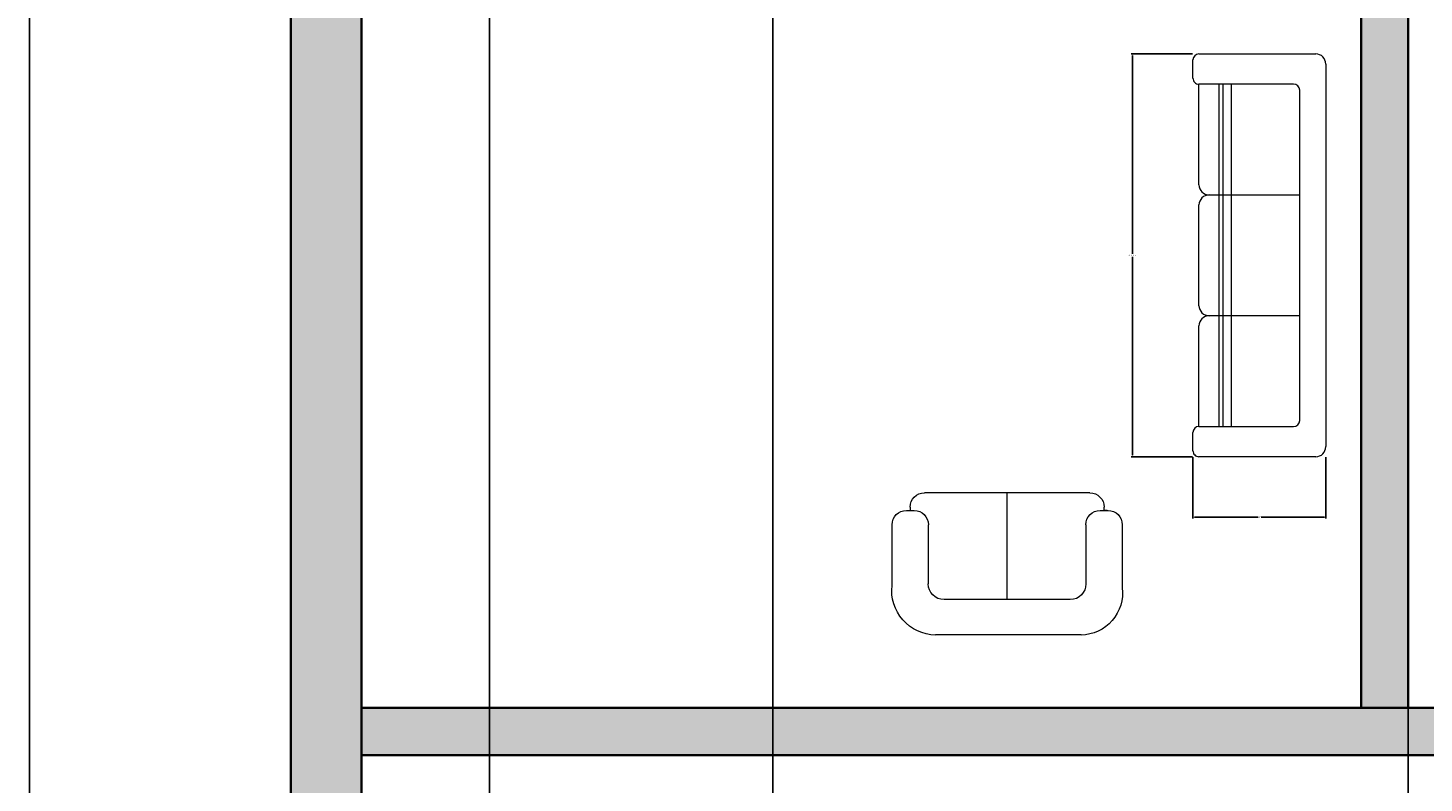
# Model space of a CAD drawing. Units: inches. Extents: x 2070 to 4408, y 1595 to 4269.
# Tile 2 of 20: x 2070 to 2247, y 1739 to 1835. Entities that reach past the tile are written whole.
import ezdxf

# ---------------------------------------------------------------- set-up
doc = ezdxf.new("R2010")
doc.units = ezdxf.units.IN
for name, color, linetype, lineweight in [('A-ANNO-DIMS', 2, 'Continuous', 18), ('A-FURN', 8, 'Continuous', 18), ('A-WALL', 7, 'Continuous', 35)]:
    doc.layers.add(name, color=color, linetype=linetype, lineweight=lineweight)
doc.layers.add('A-WALL-PATT', color=18, linetype='Continuous', lineweight=13, true_color=0x000000)
doc.styles.get("Standard").update_dxf_attribs({"font": 'arial.ttf'})
doc.dimstyles.get("Standard").update_dxf_attribs({"dimtxt": 0.18, "dimasz": 0.18, "dimexe": 0.18, "dimexo": 0.0625, "dimgap": 0.09, "dimtad": 0, "dimtih": 1, "dimtoh": 1, "dimdec": 4, "dimzin": 0, "dimdsep": 46, "dimtxsty": 'Standard', "dimcen": 0.09, "dimadec": 0, "dimazin": 0, "dimtfac": 1, "dimtdec": 4, "dimtofl": 0, "dimtmove": 0, "dimatfit": 3, "dimfxl": 1, "dimtolj": 1, "dimtzin": 0, "dimarcsym": 0})

# ---------------------------------------------------------------- blocks, each defined once
blk = doc.blocks.new('A$C05BA3A2B')
for p, q in [((0.05, 0.6596), (1.95, 0.6596)), ((0.05, 0.6596), (1.95, 0.6596)), ((0.05, 0.6596), (1.95, 0.6596)), ((0, 0.03), (0, 0.6096)), ((0, 0.03), (0, 0.6096)), ((0, 0.03), (0, 0.6096)), ((2, 0.6096), (2, 0.03)), ((2, 0.6096), (2, 0.03)), ((2, 0.6096), (2, 0.03)), ((0.15, 0.5), (0.15, 0.03)), ((0.15, 0.5), (0.15, 0.03)), ((0.15, 0.5), (0.15, 0.03)), ((1.82, 0.53), (0.18, 0.53)), ((1.82, 0.53), (0.18, 0.53)), ((1.82, 0.53), (0.18, 0.53)), ((0.7, 0.08), (0.7, 0.53)), ((0.7, 0.08), (0.7, 0.53)), ((0.7, 0.08), (0.7, 0.53)), ((1.3, 0.53), (1.3, 0.08)), ((1.3, 0.53), (1.3, 0.08)), ((1.3, 0.53), (1.3, 0.08)), ((1.85, 0.03), (1.85, 0.5)), ((1.85, 0.03), (1.85, 0.5)), ((1.85, 0.03), (1.85, 0.5)), ((1.85, 0.1908), (0.15, 0.1908)), ((1.85, 0.1908), (0.15, 0.1908)), ((1.85, 0.1908), (0.15, 0.1908)), ((1.85, 0.1508), (0.15, 0.1508)), ((1.85, 0.1508), (0.15, 0.1508)), ((1.85, 0.1508), (0.15, 0.1508)), ((1.85, 0.1308), (0.15, 0.1308)), ((1.85, 0.1308), (0.15, 0.1308)), ((1.85, 0.1308), (0.15, 0.1308)), ((0.12, 0), (0.03, 0)), ((0.12, 0), (0.03, 0)), ((0.12, 0), (0.03, 0)), ((0.65, 0.03), (0.15, 0.03)), ((0.65, 0.03), (0.15, 0.03)), ((0.65, 0.03), (0.15, 0.03)), ((1.25, 0.03), (0.75, 0.03)), ((1.25, 0.03), (0.75, 0.03)), ((1.25, 0.03), (0.75, 0.03)), ((1.85, 0.03), (1.35, 0.03)), ((1.85, 0.03), (1.35, 0.03)), ((1.85, 0.03), (1.35, 0.03)), ((1.97, 0), (1.88, 0)), ((1.97, 0), (1.88, 0)), ((1.97, 0), (1.88, 0))]:
    blk.add_line(p, q)
for centre, radius, start, end in [((0.05, 0.6096), 0.05, 90, 180), ((0.05, 0.6096), 0.05, 90, 180), ((0.05, 0.6096), 0.05, 90, 180), ((1.95, 0.6096), 0.05, 0, 90), ((1.95, 0.6096), 0.05, 0, 90), ((1.95, 0.6096), 0.05, 0, 90), ((0.18, 0.5), 0.03, 90, 180), ((0.18, 0.5), 0.03, 90, 180), ((0.18, 0.5), 0.03, 90, 180), ((1.82, 0.5), 0.03, 0, 90), ((1.82, 0.5), 0.03, 0, 90), ((1.82, 0.5), 0.03, 0, 90), ((0.65, 0.08), 0.05, 270, 0), ((0.65, 0.08), 0.05, 270, 0), ((0.65, 0.08), 0.05, 270, 0), ((0.75, 0.08), 0.05, 180, 270), ((0.75, 0.08), 0.05, 180, 270), ((0.75, 0.08), 0.05, 180, 270), ((1.25, 0.08), 0.05, 270, 0), ((1.25, 0.08), 0.05, 270, 0), ((1.25, 0.08), 0.05, 270, 0), ((1.35, 0.08), 0.05, 180, 270), ((1.35, 0.08), 0.05, 180, 270), ((1.35, 0.08), 0.05, 180, 270), ((0.03, 0.03), 0.03, 180, 270), ((0.03, 0.03), 0.03, 180, 270), ((0.03, 0.03), 0.03, 180, 270), ((0.12, 0.03), 0.03, 270, 0), ((0.12, 0.03), 0.03, 270, 0), ((0.12, 0.03), 0.03, 270, 0), ((1.88, 0.03), 0.03, 180, 270), ((1.88, 0.03), 0.03, 180, 270), ((1.88, 0.03), 0.03, 180, 270), ((1.97, 0.03), 0.03, 270, 0), ((1.97, 0.03), 0.03, 270, 0), ((1.97, 0.03), 0.03, 270, 0)]:
    blk.add_arc(centre, radius, start, end)
blk = doc.blocks.new('A$C6D011943')
for p, q in [((1.448, 1.089), (0.332, 1.089)), ((1.364, 0.818), (0.398, 0.818)), ((0.881, 0.818), (0.881, 0)), ((0, 0.709), (0, 0.247)), ((0.278, 0.697), (0.278, 0.244)), ((1.485, 0.244), (1.485, 0.697)), ((1.762, 0.247), (1.762, 0.727)), ((0.109, 0.136), (0.169, 0.136)), ((0.139, 0.109), (0.139, 0.136)), ((1.593, 0.136), (1.654, 0.136)), ((1.648, 0.136), (1.623, 0.136)), ((1.623, 0.109), (1.623, 0.136)), ((1.515, 0), (0.247, 0))]:
    blk.add_line(p, q)
for centre, radius, start, end in [((0.339, 0.748), 0.342, 91.2564, 186.501), ((1.441, 0.766), 0.324, 353.159, 88.6697), ((0.398, 0.697), 0.121, 90, 180), ((1.364, 0.697), 0.121, 0, 90), ((0.109, 0.244), 0.109, 180, 270), ((0.169, 0.244), 0.109, 270, 0), ((1.593, 0.244), 0.109, 180, 270), ((1.654, 0.244), 0.109, 270, 0), ((0.247, 0.109), 0.109, 180, 270), ((1.515, 0.109), 0.109, 270, 0)]:
    blk.add_arc(centre, radius, start, end)
blk = doc.blocks.new('*D19')
at = {"layer": 'A-ANNO-DIMS', "color": 0, "lineweight": -2, "transparency": 16777216}
for p, q in [((2217.78, 1831.51), (2209.98, 1831.51)), ((2210.16, 1831.33), (2210.16, 1806.1)), ((2210.16, 1780.51), (2210.16, 1805.73)), ((2217.78, 1780.33), (2209.98, 1780.33))]:
    blk.add_line(p, q, dxfattribs=at)
at = {"layer": 'A-ANNO-DIMS', "color": 0, "transparency": 16777216}
for points in [[(2210.13, 1831.33), (2210.19, 1831.33), (2210.16, 1831.51)], [(2210.13, 1780.51), (2210.19, 1780.51), (2210.16, 1780.33)]]:
    blk.add_solid(points, dxfattribs=at)
at = {"layer": 'Defpoints', "color": 0, "transparency": 16777216}
for p in [(2217.84, 1831.51), (2210.16, 1780.33), (2217.84, 1780.33)]:
    blk.add_point(p, dxfattribs=at)
at = {"layer": 'A-ANNO-DIMS', "color": 0, "transparency": 16777216, "insert": (2210.16, 1805.92), "char_height": 0.18, "attachment_point": 5}
blk.add_mtext('\\A1;SETTEE 51', dxfattribs=at)
blk = doc.blocks.new('*D20')
at = {"layer": 'A-ANNO-DIMS', "color": 0, "lineweight": -2, "transparency": 16777216}
for p, q in [((2217.84, 1780.26), (2217.84, 1772.47)), ((2234.72, 1780.26), (2234.72, 1772.47)), ((2218.02, 1772.65), (2226.07, 1772.65)), ((2234.54, 1772.65), (2226.49, 1772.65))]:
    blk.add_line(p, q, dxfattribs=at)
at = {"layer": 'A-ANNO-DIMS', "color": 0, "transparency": 16777216}
for points in [[(2218.02, 1772.68), (2218.02, 1772.62), (2217.84, 1772.65)], [(2234.54, 1772.68), (2234.54, 1772.62), (2234.72, 1772.65)]]:
    blk.add_solid(points, dxfattribs=at)
at = {"layer": 'Defpoints', "color": 0, "transparency": 16777216}
for p in [(2217.84, 1780.33), (2234.72, 1780.33), (2234.72, 1772.65)]:
    blk.add_point(p, dxfattribs=at)
at = {"layer": 'A-ANNO-DIMS', "color": 0, "transparency": 16777216, "insert": (2226.28, 1772.65), "char_height": 0.18, "attachment_point": 5}
blk.add_mtext('\\A1;17', dxfattribs=at)
blk = doc.blocks.new('*D24')
at = {"layer": 'A-ANNO-DIMS', "color": 0, "lineweight": -2, "transparency": 16777216}
for p, q in [((2103.13, 2291.4), (2069.84, 2291.4)), ((2070.02, 2291.22), (2070.02, 1960.08)), ((2070.02, 1628.58), (2070.02, 1959.72)), ((2336.13, 1628.4), (2069.84, 1628.4))]:
    blk.add_line(p, q, dxfattribs=at)
at = {"layer": 'A-ANNO-DIMS', "color": 0, "transparency": 16777216}
for points in [[(2069.99, 2291.22), (2070.05, 2291.22), (2070.02, 2291.4)], [(2069.99, 1628.58), (2070.05, 1628.58), (2070.02, 1628.4)]]:
    blk.add_solid(points, dxfattribs=at)
at = {"layer": 'Defpoints', "color": 0, "transparency": 16777216}
for p in [(2070.02, 2291.4), (2103.2, 2291.4), (2336.2, 1628.4)]:
    blk.add_point(p, dxfattribs=at)
at = {"layer": 'A-ANNO-DIMS', "color": 0, "transparency": 16777216, "insert": (2070.02, 1959.9), "char_height": 0.18, "attachment_point": 5}
blk.add_mtext('\\A1;663', dxfattribs=at)
blk = doc.blocks.new('*D29')
at = {"layer": 'A-ANNO-DIMS', "color": 0, "lineweight": -2, "transparency": 16777216}
for p, q in [((2128.44, 2150.34), (2128.44, 1595.04)), ((2164.44, 2150.34), (2164.44, 1595.04)), ((2128.62, 1595.22), (2146.22, 1595.22)), ((2164.26, 1595.22), (2146.65, 1595.22))]:
    blk.add_line(p, q, dxfattribs=at)
at = {"layer": 'A-ANNO-DIMS', "color": 0, "transparency": 16777216}
for points in [[(2128.62, 1595.25), (2128.62, 1595.19), (2128.44, 1595.22)], [(2164.26, 1595.25), (2164.26, 1595.19), (2164.44, 1595.22)]]:
    blk.add_solid(points, dxfattribs=at)
at = {"layer": 'Defpoints', "color": 0, "transparency": 16777216}
for p in [(2128.44, 2150.4), (2164.44, 2150.4), (2164.44, 1595.22)]:
    blk.add_point(p, dxfattribs=at)
at = {"layer": 'A-ANNO-DIMS', "color": 0, "transparency": 16777216, "insert": (2146.44, 1595.22), "char_height": 0.18, "attachment_point": 5}
blk.add_mtext('\\A1;36', dxfattribs=at)
blk = doc.blocks.new('*D32')
at = {"layer": 'A-ANNO-DIMS', "color": 0, "lineweight": -2, "transparency": 16777216}
for p, q in [((2245.2, 2230.58), (2245.2, 1595.04)), ((2340.2, 2230.58), (2340.2, 1595.04)), ((2245.38, 1595.22), (2292.48, 1595.22)), ((2340.02, 1595.22), (2292.92, 1595.22))]:
    blk.add_line(p, q, dxfattribs=at)
at = {"layer": 'A-ANNO-DIMS', "color": 0, "transparency": 16777216}
for points in [[(2245.38, 1595.25), (2245.38, 1595.19), (2245.2, 1595.22)], [(2340.02, 1595.25), (2340.02, 1595.19), (2340.2, 1595.22)]]:
    blk.add_solid(points, dxfattribs=at)
at = {"layer": 'Defpoints', "color": 0, "transparency": 16777216}
for p in [(2245.2, 2230.65), (2340.2, 2230.65), (2340.2, 1595.22)]:
    blk.add_point(p, dxfattribs=at)
at = {"layer": 'A-ANNO-DIMS', "color": 0, "transparency": 16777216, "insert": (2292.7, 1595.22), "char_height": 0.18, "attachment_point": 5}
blk.add_mtext('\\A1;95', dxfattribs=at)

msp = doc.modelspace()

# ---------------------------------------------------------------- hatches: boundary and pattern name
at = {"layer": 'A-WALL-PATT'}
h = msp.add_hatch(color=256, dxfattribs=at)
h.dxf.hatch_style = 1
h.paths.add_polyline_path([(2346.196, 2218.3995), (2346.196, 2282.3995), (2340.196, 2282.3995), (2340.196, 2212.3995), (2345.5866, 2212.3995), (2346.196, 2212.3995)], flags=0)
h.paths.add_polyline_path([(2245.196, 2282.3995), (2239.196, 2282.3995), (2239.196, 2186.3995), (2244.5866, 2186.3995), (2245.196, 2186.3995)], flags=0)
h.paths.add_polyline_path([(2340.196, 2230.6455), (2245.196, 2230.6455), (2245.196, 2224.6455), (2340.196, 2224.6455)], flags=0)
h.paths.add_polyline_path([(2245.196, 2150.3995), (2239.196, 2150.3995), (2164.4362, 2150.3995), (2164.4362, 2144.3995), (2239.196, 2144.3995), (2239.196, 2086.3995), (2239.196, 2067.2711), (2244.5866, 2067.2711), (2245.196, 2067.2711), (2245.196, 2144.3995)], flags=0)
h.paths.add_polyline_path([(2346.196, 2176.3995), (2340.196, 2176.3995), (2340.196, 2086.3995), (2346.196, 2086.3995), (2346.196, 2125.318)], flags=0)
h.paths.add_polyline_path([(2446.196, 2086.3995), (2346.196, 2086.3995), (2340.196, 2086.3995), (2340.196, 2080.3995), (2446.196, 2080.3995)], flags=0)
h.paths.add_polyline_path([(2455.196, 2291.3995), (2103.196, 2291.3995), (2103.196, 1699.3995), (2336.196, 1699.3995), (2336.196, 1628.3995), (2345.196, 1628.3995), (2446.196, 1628.3995), (2454.8846, 1628.3995), (2454.8846, 1699.3995)])
h.paths.add_polyline_path([(2446.196, 2282.3995), (2446.196, 2218.3995), (2446.196, 2212.3995), (2446.196, 2086.3995), (2446.196, 2080.3995), (2446.196, 1708.3995), (2446.196, 1637.3995), (2345.196, 1637.3995), (2345.196, 1699.3995), (2345.196, 1708.3995), (2336.196, 1708.3995), (2112.196, 1708.3995), (2112.196, 2282.3995), (2239.196, 2282.3995), (2245.196, 2282.3995), (2356.196, 2282.3995)], flags=16)
h.paths.add_polyline_path([(2245.196, 2150.3995), (2245.196, 2144.3995), (2245.196, 2067.2711), (2244.5866, 2067.2711), (2239.196, 2067.2711), (2239.196, 2065.6988), (2203.2929, 2065.6988, 0.40145271), (2239.196, 2031.3337), (2244.5866, 2031.3337), (2245.196, 2031.2711), (2245.196, 1924.1525), (2239.196, 1924.1525), (2239.196, 1922.5803), (2203.2929, 1922.5803, 0.40145271), (2239.196, 1888.2151), (2244.5866, 1888.2151), (2245.196, 1888.1525), (2245.196, 1748.3995), (2339.196, 1748.4621, -0.40145271), (2303.2929, 1782.8272), (2303.2585, 1782.8272), (2303.2585, 1784.3995), (2339.196, 1784.3995), (2339.196, 1877.2067), (2291.196, 1877.2067), (2291.196, 1883.2067), (2291.196, 1946.3995), (2291.196, 1952.3995), (2291.196, 2086.3995), (2297.196, 2086.3995), (2302.196, 2086.3995), (2302.196, 2081.0259), (2303.7633, 2081.0259), (2303.7633, 2080.3995), (2338.0148, 2080.3995, 0.00437129), (2338.0203, 2081.0259), (2338.0203, 2086.3995), (2340.196, 2086.3995), (2340.196, 2176.4621), (2345.5866, 2176.4621, 0.40145271), (2381.4896, 2210.8272), (2345.5866, 2210.8272), (2345.5866, 2212.3995), (2340.196, 2212.3995), (2340.196, 2224.6455), (2245.196, 2224.6455), (2245.196, 2186.3995), (2244.5866, 2186.3995), (2239.196, 2186.3995), (2239.196, 2184.8272), (2203.2929, 2184.8272, 0.40145271), (2239.196, 2150.4621), (2244.5866, 2150.4621)], flags=0)
h.paths.add_polyline_path([(2346.196, 2282.3995), (2346.196, 2218.3995), (2377.1813, 2218.3995), (2377.1813, 2212.3995), (2346.196, 2212.3995), (2345.5866, 2212.3995), (2340.196, 2212.3995), (2340.196, 2224.6455), (2245.196, 2224.6455), (2245.196, 2230.6455), (2245.196, 2282.3995), (2292.696, 2256.5225), (2340.196, 2282.3995)], flags=0)
h.paths.add_polyline_path([(2346.196, 2086.3995), (2340.196, 2086.3995), (2340.196, 2080.3995), (2446.196, 2080.3995), (2431.196, 2016.3995), (2446.196, 1952.3995), (2412.196, 1952.3995), (2412.196, 2080.3995), (2340.196, 2080.3995), (2340.196, 2086.3995), (2340.196, 2176.3995), (2346.196, 2176.3995), (2346.196, 2125.318)], flags=0)
h.paths.add_polyline_path([(2186.508, 2270.0471, -0.03755288), (2186.9712, 2269.8581), (2186.9164, 2270.112, -0.02759121)], flags=0)
h.paths.add_polyline_path([(2183.955, 2273.7766, 1), (2188.2945, 2273.7766, 1)], flags=0)
h.paths.add_polyline_path([(2142.5261, 2274.6158, -0.03707541), (2142.5672, 2275.1696), (2142.5672, 2276.826), (2119.8759, 2276.826), (2119.8759, 2263.0962), (2140.4332, 2263.0962), (2142.5672, 2263.0962), (2142.5672, 2274.0621, -0.03707541)], flags=0)
h.paths.add_polyline_path([(2209.8974, 2263.0962), (2209.8974, 2262.2079), (2190.8042, 2262.2079), (2190.8042, 2263.0962)], flags=0)
h.paths.add_polyline_path([(2210.6382, 2276.1833), (2210.6382, 2263.9844), (2190.2185, 2263.9844), (2190.2185, 2276.1833)], flags=0)
h.paths.add_polyline_path([(2188.4362, 2273.7766, -1), (2183.8133, 2273.7766, -1)], flags=0)
h.paths.add_polyline_path([(2245.196, 2150.3995), (2245.196, 2144.3995), (2245.196, 2067.2711), (2239.196, 2067.2711), (2239.196, 2080.3995), (2172.196, 2080.3995), (2172.196, 2000.3995), (2239.196, 2000.3995), (2239.196, 1940.3995), (2159.0187, 1940.3995), (2123.0187, 1940.3995), (2112.196, 1940.3995), (2112.196, 1946.3995), (2123.0187, 1946.3995), (2123.0187, 1982.2238), (2124.586, 1982.2238), (2124.586, 1982.1895, -0.40145271), (2158.8429, 1946.3995), (2159.0187, 1946.3995), (2239.196, 1946.3995), (2239.196, 1994.3995), (2112.196, 1994.3995), (2112.196, 2000.3995), (2139.196, 2040.3995), (2112.196, 2080.3995), (2112.196, 2086.3995), (2239.196, 2086.3995), (2239.196, 2144.3995), (2209.5809, 2144.3995), (2209.5809, 2136.3995), (2203.0809, 2136.3995), (2205.0809, 2130.3996, -0.70257121), (2199.081, 2116.3995, -0.70256205), (2193.0809, 2130.3994), (2195.0809, 2136.3995), (2192.0809, 2136.3995), (2192.0809, 2134.8995), (2189.0809, 2134.8995), (2189.0809, 2135.8995), (2191.0809, 2135.8995), (2191.0809, 2136.3995), (2188.5809, 2136.3995), (2188.5809, 2144.3995), (2164.2481, 2144.3995, -0.39385849), (2130.0035, 2109.5491), (2130.0035, 2109.5147), (2128.4362, 2109.5147), (2128.4362, 2144.3995), (2112.196, 2144.3995), (2112.196, 2150.3995), (2128.4362, 2150.3995), (2128.4362, 2150.7127), (2164.4362, 2150.7127), (2164.4362, 2150.3995), (2239.196, 2150.3995)], flags=0)
h.paths.add_polyline_path([(2188.2075, 2266.8735), (2188.2075, 2211.8632, -0.41421356), (2185.4833, 2209.1391), (2146.7995, 2209.1391, -0.41421356), (2144.0754, 2211.8632), (2144.0754, 2266.8735, -0.41421356), (2146.7995, 2269.5976), (2185.4833, 2269.5976, -0.41421356)], flags=0)
h.paths.add_polyline_path([(2185.0844, 2273.7766, -1), (2187.1651, 2273.7766, -1)], flags=0)
h.paths.add_polyline_path([(2182.0486, 2259.2932), (2168.0953, 2259.2932), (2168.0953, 2260.8424), (2163.7261, 2260.8424), (2163.7261, 2259.2932), (2149.7727, 2259.2932), (2149.7727, 2266.3352), (2163.7261, 2266.3352), (2163.7261, 2261.9839), (2168.0953, 2261.9839), (2168.0953, 2266.3352), (2182.0486, 2266.3352)], flags=0)
h.paths.add_polyline_path([(2148.2585, 2250.2051), (2153.0615, 2241.8861, 0.39807048)], flags=0)
h.paths.add_polyline_path([(2162.7572, 2247.2885), (2153.1461, 2241.7396), (2148.1083, 2250.4653), (2157.7194, 2256.0142)], flags=0)
h.paths.add_polyline_path([(2162.6726, 2247.4351, -0.39286196), (2157.8415, 2255.6313), (2157.6431, 2255.6313), (2157.8696, 2255.7541)], flags=0)
h.paths.add_polyline_path([(2164.2604, 2145.339), (2164.4362, 2144.3995), (2164.4362, 2150.3995), (2164.2604, 2150.7127)], flags=0)
h.paths.add_polyline_path([(2208.5809, 2142.6495), (2208.5809, 2138.3995, -0.41421356), (2207.8309, 2137.3995), (2190.5809, 2137.3995, -0.41421356), (2189.5809, 2138.1495), (2189.5809, 2142.3995, -0.41421356), (2190.3309, 2143.3995), (2207.5809, 2143.3995, -0.41421356)], flags=0)
h.paths.add_polyline_path([(2147.957, 2229.9119), (2154.7494, 2223.1195, 0.39807048)], flags=0)
h.paths.add_polyline_path([(2162.7165, 2230.8473), (2154.8691, 2222.9998), (2147.7446, 2230.1244), (2155.592, 2237.9718)], flags=0)
h.paths.add_polyline_path([(2162.5969, 2230.9669, -0.39807048), (2155.8044, 2237.7594)], flags=0)
h.paths.add_polyline_path([(2391.8776, 2049.9192), (2408.5766, 2049.9192), (2408.5766, 2033.2202), (2408.5766, 1983.123), (2408.5766, 1966.4239), (2391.8776, 1966.4239), (2391.8776, 1983.123), (2341.7804, 1983.123), (2341.7804, 2033.2202), (2391.8776, 2033.2202)], flags=0)
h.paths.add_polyline_path([(2144.1055, 2274.6158, 1), (2148.445, 2274.6158, 1)], flags=0)
h.paths.add_polyline_path([(2148.5867, 2274.6158, -1), (2143.9638, 2274.6158, -1)], flags=0)
h.paths.add_polyline_path([(2145.2349, 2274.6158, -1), (2147.3156, 2274.6158, -1)], flags=0)
edge = h.paths.add_edge_path(flags=0)
edge.add_ellipse((2400.5951, 2040.9436), major_axis=(-4.5109, 0), ratio=0.97544784, start_angle=180, end_angle=270, ccw=False)
edge.add_ellipse((2400.5951, 2040.9436), major_axis=(-4.5109, 0), ratio=0.97544784, start_angle=90, end_angle=180, ccw=False)
edge.add_ellipse((2400.5951, 2040.9436), major_axis=(-4.5109, 0), ratio=0.97544784, start_angle=0, end_angle=90, ccw=False)
edge.add_ellipse((2400.5951, 2040.9436), major_axis=(-4.5109, 0), ratio=0.97544784, start_angle=270, end_angle=360, ccw=False)
h.paths.add_polyline_path([(2199.0809, 2117.3995, -0.73452973), (2195.0809, 2130.3995), (2203.081, 2130.3995, -0.73453329)], flags=0)
h.paths.add_polyline_path([(2141.9147, 2276.0353), (2141.9147, 2263.9844), (2120.4685, 2263.9844), (2120.4685, 2276.0353)], flags=0)
h.paths.add_polyline_path([(2138.4481, 2273.4072), (2138.4481, 2266.7226), (2133.2801, 2266.7226), (2133.2801, 2273.4072)], flags=0)
h.paths.add_polyline_path([(2137.9691, 2272.9175), (2137.9691, 2272.204), (2135.4229, 2272.204), (2135.4229, 2271.6329), (2135.3221, 2270.1051), (2135.3221, 2269.0265), (2135.4229, 2268.6811), (2135.4229, 2267.2011), (2133.7212, 2267.2011), (2133.7212, 2268.6811), (2133.7983, 2269.9587), (2133.7983, 2271.2758), (2133.7212, 2271.6329), (2133.7212, 2273.0065), (2135.717, 2273.0065), (2135.717, 2272.9175)], flags=0)
h.paths.add_polyline_path([(2137.9215, 2271.8264), (2137.9215, 2271.3786), (2137.5182, 2271.3786), (2136.9355, 2271.3786), (2136.3529, 2271.3786), (2135.7703, 2271.3786), (2135.7703, 2271.8264), (2136.1736, 2271.8264), (2136.7562, 2271.8264), (2137.3389, 2271.8264)], flags=0)
h.paths.add_polyline_path([(2137.9215, 2271.692), (2137.5182, 2271.692), (2136.9355, 2271.513), (2137.3389, 2271.513)], flags=0)
h.paths.add_polyline_path([(2136.3529, 2271.692), (2135.7703, 2271.513), (2136.1736, 2271.513), (2136.7562, 2271.692)], flags=0)
h.paths.add_polyline_path([(2137.9215, 2271.513), (2137.5182, 2271.513), (2136.7562, 2271.747), (2136.7562, 2271.692), (2137.3389, 2271.692)], flags=0)
h.paths.add_polyline_path([(2137.8207, 2270.4664), (2137.8207, 2270.0971), (2137.8207, 2269.627), (2137.8207, 2269.1569), (2137.8207, 2268.6868), (2137.3837, 2268.6868), (2136.6442, 2268.6868), (2135.9271, 2268.6868), (2135.9271, 2269.0562), (2135.9271, 2269.5263), (2135.9271, 2269.9963), (2135.9271, 2270.4664), (2136.3641, 2270.4664), (2137.0812, 2270.4664)], flags=0)
h.paths.add_polyline_path([(2137.3837, 2269.627), (2137.8207, 2269.627), (2137.8207, 2269.5263), (2137.3837, 2269.5263), (2137.3837, 2269.1569), (2137.8207, 2269.1569), (2137.3837, 2269.0562), (2137.3837, 2268.6868), (2137.0812, 2268.6868), (2137.0812, 2269.0562), (2136.6442, 2269.0562), (2136.6442, 2268.6868), (2136.3641, 2268.6868), (2136.3641, 2269.0562), (2135.9271, 2269.0562), (2135.9271, 2269.1569), (2136.3641, 2269.1569), (2136.3641, 2269.5263), (2135.9271, 2269.5263), (2135.9271, 2269.627), (2136.3641, 2269.627), (2136.3641, 2269.9963), (2135.9271, 2269.9963), (2136.3641, 2270.0971), (2136.3641, 2270.4664), (2136.6442, 2270.4664), (2136.6442, 2270.0971), (2137.0812, 2270.0971), (2137.0812, 2270.4664), (2137.3837, 2270.4664), (2137.3837, 2270.0971), (2137.8207, 2270.0971), (2137.3837, 2269.9963)], flags=0)
h.paths.add_polyline_path([(2137.5182, 2271.8264), (2137.5182, 2271.692), (2137.3389, 2271.3786), (2137.3389, 2271.513)], flags=0)
h.paths.add_polyline_path([(2137.8179, 2267.8138), (2137.8179, 2267.6879), (2137.1876, 2267.6879), (2136.4733, 2267.6879), (2135.759, 2267.6879), (2135.759, 2267.8138), (2136.3893, 2267.8138), (2137.1036, 2267.8138)], flags=0)
h.paths.add_polyline_path([(2137.0812, 2269.9963), (2137.0812, 2269.627), (2137.0812, 2269.1569), (2136.6442, 2269.1569), (2136.6442, 2269.5263), (2136.6442, 2269.9963)], flags=0)
h.paths.add_polyline_path([(2136.3529, 2271.8264), (2136.3529, 2271.692), (2136.1736, 2271.3786), (2136.1736, 2271.513)], flags=0)
h.paths.add_polyline_path([(2136.4733, 2267.8138), (2136.4733, 2267.6879), (2136.3893, 2267.6879), (2136.3893, 2267.8138)], flags=0)
h.paths.add_polyline_path([(2407.9087, 2032.5522), (2407.9087, 1983.7909), (2359.81, 1983.7909, -0.00912788), (2359.0575, 1983.7909), (2342.4483, 1983.7909), (2342.4483, 2032.5522)], flags=0)
h.paths.add_polyline_path([(2389.1838, 2023.1358), (2353.7856, 2023.1358), (2353.7856, 1985.4867, -0.09210376), (2350.2788, 1988.655), (2350.2788, 2026.6426), (2389.1838, 2026.6426)], flags=0)
h.paths.add_polyline_path([(2352.6166, 2024.3048), (2351.4477, 2024.3048), (2351.4477, 2025.4737), (2352.6166, 2025.4737)], flags=0)
h.paths.add_polyline_path([(2399.6319, 2026.7589), (2404.3661, 2026.7589, -0.41421356), (2407.0379, 2024.087), (2407.0379, 2013.4908, -0.41421356), (2404.3661, 2010.819), (2399.6319, 2010.819, -0.41421356), (2396.96, 2013.4908), (2396.96, 2024.087, -0.41421356)], flags=0)
h.paths.add_polyline_path([(2399.6319, 2026.0909), (2404.3661, 2026.0909, -0.41421356), (2406.37, 2024.087), (2406.37, 2013.4908, -0.41421356), (2404.3661, 2011.487), (2399.6319, 2011.487, -0.41421356), (2397.628, 2013.4908), (2397.628, 2024.087, -0.41421356)], flags=0)
h.paths.add_polyline_path([(2399.6319, 2002.3217), (2404.3661, 2002.3217, -0.41421356), (2407.0379, 1999.6498), (2407.0379, 1989.0536, -0.41421356), (2404.3661, 1986.3818), (2399.6319, 1986.3818, -0.41421356), (2396.96, 1989.0536), (2396.96, 1999.6498, -0.41421356)], flags=0)
h.paths.add_polyline_path([(2399.6319, 2001.6537), (2404.3661, 2001.6537, -0.41421356), (2406.37, 1999.6498), (2406.37, 1989.0536, -0.41421356), (2404.3661, 1987.0497), (2399.6319, 1987.0497, -0.41421356), (2397.628, 1989.0536), (2397.628, 1999.6498, -0.41421356)], flags=0)
edge = h.paths.add_edge_path(flags=0)
edge.add_ellipse((2400.5951, 1975.3996), major_axis=(-4.5109, 0), ratio=0.97544784, start_angle=-180, end_angle=-90, ccw=False)
edge.add_ellipse((2400.5951, 1975.3996), major_axis=(-4.5109, 0), ratio=0.97544784, start_angle=90, end_angle=180, ccw=False)
edge.add_ellipse((2400.5951, 1975.3996), major_axis=(-4.5109, 0), ratio=0.97544784, start_angle=0, end_angle=90, ccw=False)
edge.add_ellipse((2400.5951, 1975.3996), major_axis=(-4.5109, 0), ratio=0.97544784, start_angle=-90, end_angle=0, ccw=False)
h.paths.add_polyline_path([(2345.196, 1910.3995), (2366.4386, 1910.3995), (2366.4386, 1925.4555), (2392.3856, 1925.4555), (2392.3856, 1933.5025), (2400.1399, 1925.4555), (2392.3856, 1919.8795), (2392.3856, 1925.4555), (2366.4386, 1925.4555), (2366.4386, 1910.3995), (2381.196, 1910.3995), (2405.196, 1910.3995), (2405.196, 1898.3995), (2446.196, 1898.3995), (2446.196, 1886.3995), (2405.196, 1886.3995), (2405.196, 1874.3995), (2446.196, 1874.3995), (2446.196, 1862.3995), (2405.196, 1862.3995), (2405.196, 1850.3995), (2446.196, 1850.3995), (2446.196, 1838.3995), (2405.196, 1838.3995), (2405.196, 1826.3995), (2446.196, 1826.3995), (2446.196, 1814.3995), (2405.196, 1814.3995), (2405.196, 1802.3995), (2446.196, 1802.3995), (2446.196, 1798.3995), (2446.196, 1792.3995), (2405.196, 1792.3995), (2405.196, 1910.3995), (2381.196, 1910.3995), (2381.196, 1792.3995), (2345.196, 1792.3995)], flags=0)
h.paths.add_polyline_path([(2333.0944, 1863.3993, -0.41421356), (2334.7225, 1861.7712), (2334.7225, 1859.329), (2335.2653, 1859.329, -0.41421356), (2337.4361, 1857.1582), (2337.4361, 1843.862, -0.41421356), (2335.2653, 1841.6911, -0.41421356), (2337.4361, 1839.5203), (2337.4361, 1827.5808, -0.41421356), (2335.2653, 1825.41, -0.41421356), (2337.4361, 1823.2392), (2337.4361, 1808.5862, -0.41421356), (2335.2653, 1806.4153), (2334.7225, 1806.4153), (2334.7225, 1803.9732, -0.41421356), (2333.0944, 1802.3451), (2317.356, 1802.3451), (2317.0846, 1802.3451, -0.41421356), (2315.7279, 1803.7018), (2315.7279, 1803.8646), (2313.8284, 1803.8646, -0.41421356), (2311.6576, 1806.0354), (2311.6576, 1823.2015, -0.39597602), (2313.6834, 1825.3765, -0.43384798), (2311.6576, 1827.2718), (2311.6576, 1839.761, -0.41421356), (2313.5571, 1841.6604), (2313.8284, 1841.6604), (2333.8159, 1841.6604, -0.04213623), (2334.1798, 1841.6911, -0.41421356), (2332.009, 1843.862), (2332.009, 1857.1582, -0.41421356), (2334.1798, 1859.329), (2317.356, 1859.329), (2317.0846, 1859.329, -0.41421356), (2315.7279, 1860.6858), (2315.7279, 1862.0426, -0.41421356), (2317.0846, 1863.3993), (2317.356, 1863.3993)], flags=0)
h.paths.add_polyline_path([(2208.8475, 1848.9818), (2208.8475, 1840.9741, -0.41421356), (2207.0458, 1839.1724), (2206.5453, 1839.1721), (2206.5453, 1838.7218, -0.40985861), (2204.7704, 1836.9203), (2183.7501, 1836.9203, -0.41858196), (2181.9216, 1838.7218), (2181.9216, 1839.1721), (2181.421, 1839.1724, -0.41421356), (2179.6193, 1840.9741), (2179.6193, 1848.6817, -0.44064415), (2185.1126, 1854.9874), (2203.3852, 1854.9874, -0.45707961)], flags=0)
h.paths.add_polyline_path([(2204.243, 1848.4815), (2204.243, 1848.4815, 0.41725335), (2202.2204, 1850.4833), (2186.2049, 1850.4833, 0.4111805), (2184.2237, 1848.4815), (2184.2237, 1848.4815, -0.4111807), (2186.2049, 1850.4833), (2202.2204, 1850.4833, -0.41725315)], flags=0)
h.paths.add_polyline_path([(2234.7177, 1830.228), (2234.7176, 1781.6047, -0.41421356), (2233.4381, 1780.3252), (2218.6064, 1780.3252, -0.41421356), (2217.8387, 1781.0929), (2217.8387, 1783.3961, -0.41421356), (2218.6064, 1784.1639), (2218.6065, 1796.9595, -0.41421356), (2219.886, 1798.239, -0.41421356), (2218.6065, 1799.5186), (2218.6065, 1812.3142, -0.41421356), (2219.8861, 1813.5938, -0.41421356), (2218.6065, 1814.8733), (2218.6065, 1827.6689, -0.41421356), (2217.8388, 1828.4367), (2217.8388, 1830.7399, -0.41421356), (2218.6065, 1831.5076), (2233.4382, 1831.5076, -0.41421356)], flags=0)
h.paths.add_polyline_path([(2230.6344, 1827.6689, -0.41421356), (2231.4021, 1826.9012), (2231.4021, 1784.9316, -0.41421356), (2230.6343, 1784.1639), (2221.1853, 1784.1639), (2221.1853, 1827.6689)], flags=0)
h.paths.add_polyline_path([(2222.7208, 1798.239), (2221.6971, 1798.239), (2221.6971, 1813.5938), (2222.7208, 1813.5938)], flags=0)
h.paths.add_polyline_path([(2206.5453, 1773.935), (2206.5453, 1773.4848), (2206.9457, 1773.4848), (2207.0458, 1773.4845, -0.41421356), (2208.8475, 1771.6827), (2208.8475, 1763.675, -0.44222432), (2203.6505, 1757.6695), (2185.3851, 1757.6695, -0.45508402), (2179.6193, 1763.9752), (2179.6193, 1771.6827, -0.41421356), (2181.421, 1773.4845), (2181.421, 1773.4848), (2181.9216, 1773.4848), (2181.9216, 1773.935, -0.40985861), (2183.6965, 1775.7366), (2204.7167, 1775.7366, -0.41858196)], flags=0)
h.paths.add_polyline_path([(2202.2619, 1762.1736), (2186.2464, 1762.1736, -0.41725315), (2184.2237, 1764.1754), (2184.2237, 1764.1754, 0.41725335), (2186.2464, 1762.1736), (2202.2619, 1762.1736, 0.4111805), (2204.243, 1764.1754), (2204.243, 1764.1754, -0.4111807)], flags=0)
h.paths.add_polyline_path([(2313.0034, 1713.1906), (2312.997, 1713.1697), (2313.0123, 1713.1612)], flags=0)
h.paths.add_polyline_path([(2305.7314, 1721.0488), (2305.6257, 1721.1994), (2305.4853, 1721.084)], flags=0)
h.paths.add_polyline_path([(2307.5562, 1726.1427), (2307.6186, 1726.1026), (2307.5737, 1726.0477), (2308.5692, 1720.6434), (2310.5345, 1721.2985), (2310.5721, 1721.411), (2310.6958, 1721.3523), (2313.8453, 1722.4021), (2314.9351, 1723.8033), (2314.9294, 1723.9165), (2315.0028, 1723.8903), (2313.874, 1722.4389), (2313.8697, 1722.4102), (2308.5692, 1720.6434), (2308.9864, 1720.122), (2309.0665, 1720.0971), (2309.053, 1720.0387), (2310.9235, 1717.7005), (2311.4182, 1717.6259), (2311.2918, 1717.2402), (2312.0655, 1716.2731), (2312.1081, 1716.2606), (2312.0969, 1716.2339), (2308.5692, 1720.6434), (2305.2249, 1717.745), (2305.232, 1717.704), (2305.1665, 1717.6944), (2308.5692, 1720.6434)], flags=0)
h.paths.add_polyline_path([(2288.2072, 1714.3431), (2288.2008, 1714.3222), (2288.216, 1714.3137)], flags=0)
h.paths.add_polyline_path([(2280.9352, 1722.2013), (2280.8295, 1722.3519), (2280.689, 1722.2365)], flags=0)
h.paths.add_polyline_path([(2282.76, 1727.2952), (2282.8224, 1727.2551), (2282.7775, 1727.2002), (2283.773, 1721.7959), (2285.7383, 1722.451), (2285.7759, 1722.5635), (2285.8995, 1722.5048), (2289.0491, 1723.5546), (2290.1389, 1724.9558), (2290.1332, 1725.069), (2290.2065, 1725.0428), (2289.0777, 1723.5915), (2289.0735, 1723.5628), (2283.773, 1721.7959), (2284.1901, 1721.2745), (2284.2703, 1721.2496), (2284.2567, 1721.1913), (2286.1273, 1718.8531), (2286.622, 1718.7785), (2286.4956, 1718.3927), (2287.2692, 1717.4256), (2287.3119, 1717.4131), (2287.3006, 1717.3864), (2283.773, 1721.7959), (2280.4286, 1718.8975), (2280.4357, 1718.8565), (2280.3703, 1718.8469), (2283.773, 1721.7959)], flags=0)
h.paths.add_polyline_path([(2302.0672, 1721.8694), (2301.8205, 1721.8572), (2301.7578, 1722.1787), (2299.415, 1724.5215), (2299.103, 1724.4694), (2299.0662, 1724.8703)], flags=0)
h.paths.add_polyline_path([(2264.5643, 1715.4956), (2264.5579, 1715.4747), (2264.5731, 1715.4662)], flags=0)
h.paths.add_polyline_path([(2257.2923, 1723.3538), (2257.1865, 1723.5044), (2257.0461, 1723.389)], flags=0)
h.paths.add_polyline_path([(2259.117, 1728.4477), (2259.1795, 1728.4077), (2259.1345, 1728.3527), (2260.13, 1722.9484), (2262.0954, 1723.6036), (2262.133, 1723.716), (2262.2566, 1723.6573), (2265.4061, 1724.7071), (2266.4959, 1726.1083), (2266.4902, 1726.2215), (2266.5636, 1726.1953), (2265.4348, 1724.744), (2265.4305, 1724.7153), (2260.13, 1722.9484), (2260.5472, 1722.427), (2260.6273, 1722.4022), (2260.6138, 1722.3438), (2262.4843, 1720.0056), (2262.979, 1719.931), (2262.8526, 1719.5452), (2263.6263, 1718.5781), (2263.6689, 1718.5656), (2263.6577, 1718.5389), (2260.13, 1722.9484), (2256.7857, 1720.05), (2256.7928, 1720.009), (2256.7273, 1719.9994), (2260.13, 1722.9484)], flags=0)
h.paths.add_polyline_path([(2277.2709, 1723.0219), (2277.0243, 1723.0097), (2276.9616, 1723.3312), (2274.6187, 1725.6741), (2274.3067, 1725.6219), (2274.27, 1726.0228)], flags=0)
h.paths.add_polyline_path([(2253.628, 1724.1744), (2253.3814, 1724.1622), (2253.3186, 1724.4838), (2250.9758, 1726.8266), (2250.6638, 1726.7744), (2250.627, 1727.1753)], flags=0)
h.paths.add_polyline_path([(2161.9194, 1715.4956), (2161.913, 1715.4747), (2161.9282, 1715.4662)], flags=0)
h.paths.add_polyline_path([(2154.6474, 1723.3538), (2154.5416, 1723.5044), (2154.4012, 1723.389)], flags=0)
h.paths.add_polyline_path([(2162.7899, 1724.744), (2162.7856, 1724.7153), (2157.4851, 1722.9484), (2157.9023, 1722.427), (2157.9824, 1722.4022), (2157.9689, 1722.3438), (2159.8394, 1720.0056), (2160.3341, 1719.931), (2160.2078, 1719.5452), (2160.9814, 1718.5781), (2161.024, 1718.5656), (2161.0128, 1718.5389), (2157.4851, 1722.9484), (2154.1408, 1720.05), (2154.1479, 1720.009), (2154.0824, 1719.9994), (2157.4851, 1722.9484), (2156.4721, 1728.4477), (2156.5346, 1728.4077), (2156.4896, 1728.3527), (2157.4851, 1722.9484), (2159.4505, 1723.6036), (2159.4881, 1723.716), (2159.6117, 1723.6573), (2162.7612, 1724.7071), (2163.851, 1726.1083), (2163.8453, 1726.2215), (2163.9187, 1726.1953)], flags=0)
h.paths.add_polyline_path([(2150.9831, 1724.1744), (2150.7365, 1724.1622), (2150.6738, 1724.4838), (2148.3309, 1726.8266), (2148.0189, 1726.7744), (2147.9822, 1727.1753)], flags=0)
h.paths.add_polyline_path([(2132.5099, 1716.6482), (2132.5035, 1716.6272), (2132.5187, 1716.6187)], flags=0)
h.paths.add_polyline_path([(2125.2379, 1724.5064), (2125.1322, 1724.6569), (2124.9917, 1724.5415)], flags=0)
h.paths.add_polyline_path([(2133.3804, 1725.8965), (2133.3762, 1725.8678), (2128.0757, 1724.101), (2128.4928, 1723.5795), (2128.5729, 1723.5547), (2128.5594, 1723.4963), (2130.43, 1721.1581), (2130.9246, 1721.0835), (2130.7983, 1720.6977), (2131.5719, 1719.7306), (2131.6146, 1719.7181), (2131.6033, 1719.6914), (2128.0757, 1724.101), (2124.7313, 1721.2025), (2124.7384, 1721.1615), (2124.6729, 1721.1519), (2128.0757, 1724.101), (2127.0626, 1729.6002), (2127.1251, 1729.5602), (2127.0801, 1729.5052), (2128.0757, 1724.101), (2130.041, 1724.7561), (2130.0786, 1724.8685), (2130.2022, 1724.8098), (2133.3517, 1725.8597), (2134.4415, 1727.2608), (2134.4358, 1727.3741), (2134.5092, 1727.3478)], flags=0)
h.paths.add_polyline_path([(2121.5736, 1725.3269), (2121.327, 1725.3148), (2121.2643, 1725.6363), (2118.9214, 1727.9791), (2118.6094, 1727.9269), (2118.5727, 1728.3279)], flags=0)
h.paths.add_polyline_path([(2433.3904, 1646.406), (2433.384, 1646.3851), (2433.3992, 1646.3766)], flags=0)
h.paths.add_polyline_path([(2426.1184, 1654.2642), (2426.0127, 1654.4148), (2425.8722, 1654.2994)], flags=0)
h.paths.add_polyline_path([(2427.9432, 1659.3581), (2428.0056, 1659.318), (2427.9606, 1659.2631), (2428.9562, 1653.8588), (2430.9215, 1654.514), (2430.9591, 1654.6264), (2431.0827, 1654.5677), (2434.2323, 1655.6175), (2435.322, 1657.0187), (2435.3163, 1657.1319), (2435.3897, 1657.1057), (2434.2609, 1655.6544), (2434.2567, 1655.6257), (2428.9562, 1653.8588), (2429.3733, 1653.3374), (2429.4534, 1653.3126), (2429.4399, 1653.2542), (2431.3105, 1650.916), (2431.8051, 1650.8414), (2431.6788, 1650.4556), (2432.4524, 1649.4885), (2432.4951, 1649.476), (2432.4838, 1649.4493), (2428.9562, 1653.8588), (2425.6118, 1650.9604), (2425.6189, 1650.9194), (2425.5535, 1650.9098), (2428.9562, 1653.8588)], flags=0)
h.paths.add_polyline_path([(2376.63, 1645.4912), (2376.6236, 1645.4703), (2376.6388, 1645.4617)], flags=0)
h.paths.add_polyline_path([(2369.358, 1653.3494), (2369.2523, 1653.5), (2369.1118, 1653.3845)], flags=0)
h.paths.add_polyline_path([(2371.1828, 1658.4432), (2371.2452, 1658.4032), (2371.2003, 1658.3482), (2372.1958, 1652.944), (2374.1611, 1653.5991), (2374.1987, 1653.7116), (2374.3224, 1653.6528), (2377.4719, 1654.7027), (2378.5617, 1656.1038), (2378.556, 1656.2171), (2378.6293, 1656.1908), (2377.5005, 1654.7395), (2377.4963, 1654.7108), (2372.1958, 1652.944), (2372.6129, 1652.4225), (2372.6931, 1652.3977), (2372.6795, 1652.3393), (2374.5501, 1650.0011), (2375.0448, 1649.9265), (2374.9184, 1649.5407), (2375.692, 1648.5737), (2375.7347, 1648.5611), (2375.7234, 1648.5344), (2372.1958, 1652.944), (2368.8514, 1650.0456), (2368.8586, 1650.0046), (2368.7931, 1649.995), (2372.1958, 1652.944)], flags=0)
h.paths.add_polyline_path([(2404.0947, 1645.0338), (2404.0883, 1645.0128), (2404.1035, 1645.0043)], flags=0)
h.paths.add_polyline_path([(2396.8227, 1652.892), (2396.717, 1653.0425), (2396.5765, 1652.9271)], flags=0)
h.paths.add_polyline_path([(2398.6475, 1657.9858), (2398.7099, 1657.9458), (2398.665, 1657.8908), (2399.6605, 1652.4866), (2401.6258, 1653.1417), (2401.6634, 1653.2541), (2401.7871, 1653.1954), (2404.9366, 1654.2453), (2406.0264, 1655.6464), (2406.0207, 1655.7596), (2406.094, 1655.7334), (2404.9652, 1654.2821), (2404.961, 1654.2534), (2399.6605, 1652.4866), (2400.0776, 1651.9651), (2400.1578, 1651.9403), (2400.1442, 1651.8819), (2402.0148, 1649.5437), (2402.5095, 1649.4691), (2402.3831, 1649.0833), (2403.1567, 1648.1162), (2403.1994, 1648.1037), (2403.1881, 1648.077), (2399.6605, 1652.4866), (2396.3162, 1649.5881), (2396.3233, 1649.5471), (2396.2578, 1649.5375), (2399.6605, 1652.4866)], flags=0)
h.paths.add_polyline_path([(2419.4532, 1658.0857), (2422.4541, 1655.0848), (2422.2075, 1655.0726), (2422.1448, 1655.3941), (2419.8019, 1657.737), (2419.4899, 1657.6848)], flags=0)
h.paths.add_polyline_path([(2390.1575, 1656.7135), (2393.1584, 1653.7125), (2392.9118, 1653.7004), (2392.8491, 1654.0219), (2390.5063, 1656.3647), (2390.1943, 1656.3125)], flags=0)
h.paths.add_polyline_path([(2362.6928, 1657.1709), (2365.6937, 1654.1699), (2365.4471, 1654.1578), (2365.3844, 1654.4793), (2363.0416, 1656.8221), (2362.7295, 1656.77)], flags=0)
h.paths.add_polyline_path([(2419.9523, 2037.8601), (2440.2872, 2037.8601), (2440.2872, 2047.1732), (2419.9523, 2047.1732)], flags=8)
h.paths.add_polyline_path([(2370.186, 1698.9005), (2413.6287, 1698.9005), (2413.6287, 1708.0908), (2370.186, 1708.0908)], flags=8)
h.paths.add_polyline_path([(2370.1656, 1708.5185), (2430.0857, 1708.5185), (2430.0857, 1717.8316), (2370.1656, 1717.8316)], flags=8)
h.paths.add_polyline_path([(2254.1469, 1788.1883), (2302.2471, 1788.1883), (2302.2471, 1797.3786), (2254.1469, 1797.3786)], flags=8)
h.paths.add_polyline_path([(2254.1264, 1797.8063), (2326.1448, 1797.8063), (2326.1448, 1807.1194), (2254.1264, 1807.1194)], flags=8)
h.paths.add_polyline_path([(2300.08, 1914.5069), (2338.861, 1914.5069), (2338.861, 1923.6972), (2300.08, 1923.6972)], flags=8)
h.paths.add_polyline_path([(2300.0595, 1924.1249), (2331.5882, 1924.1249), (2331.5882, 1933.438), (2300.0595, 1933.438)], flags=8)
h.paths.add_polyline_path([(2176.6905, 1716.4567), (2224.1441, 1716.4567), (2224.1441, 1725.647), (2176.6905, 1725.647)], flags=8)
h.paths.add_polyline_path([(2176.67, 1726.0747), (2245.9176, 1726.0747), (2245.9176, 1735.3878), (2176.67, 1735.3878)], flags=8)
h.paths.add_polyline_path([(2339.997, 2039.7696), (2388.1034, 2039.7696), (2388.1034, 2048.9661), (2339.997, 2048.9661)], flags=8)
h.paths.add_polyline_path([(2339.9776, 2049.3928), (2388.7204, 2049.3928), (2388.7204, 2058.7059), (2339.9776, 2058.7059)], flags=8)
h.paths.add_polyline_path([(2366.0063, 2161.3825), (2409.449, 2161.3825), (2409.449, 2170.5728), (2366.0063, 2170.5728)], flags=8)
h.paths.add_polyline_path([(2365.9868, 2171.0016), (2405.879, 2171.0016), (2405.879, 2180.3085), (2365.9868, 2180.3085)], flags=8)
h.paths.add_polyline_path([(2366.0102, 2247.0726), (2407.12, 2247.0726), (2407.12, 2256.263), (2366.0102, 2256.263)], flags=8)
h.paths.add_polyline_path([(2365.9897, 2256.6906), (2397.9686, 2256.6906), (2397.9686, 2266.0037), (2365.9897, 2266.0037)], flags=8)
h.paths.add_polyline_path([(2271.8465, 2102.7885), (2307.6541, 2102.7885), (2307.6541, 2111.9849), (2271.8465, 2111.9849)], flags=8)
h.paths.add_polyline_path([(2271.8281, 2112.4126), (2304.2673, 2112.4126), (2304.2673, 2121.7196), (2271.8281, 2121.7196)], flags=8)
h.paths.add_polyline_path([(2141.6408, 2187.5934), (2182.108, 2187.5934), (2182.108, 2196.7837), (2141.6408, 2196.7837)], flags=8)
h.paths.add_polyline_path([(2141.6203, 2197.2114), (2190.3631, 2197.2114), (2190.3631, 2206.5245), (2141.6203, 2206.5245)], flags=8)
h.paths.add_polyline_path([(2165.7271, 2103.039), (2211.5027, 2103.039), (2211.5027, 2112.2293), (2165.7271, 2112.2293)], flags=8)
h.paths.add_polyline_path([(2165.7077, 2112.658), (2185.1033, 2112.658), (2185.1033, 2121.965), (2165.7077, 2121.965)], flags=8)
h.paths.add_polyline_path([(2174.945, 2048.0789), (2211.3973, 2048.0789), (2211.3973, 2057.2693), (2174.945, 2057.2693)], flags=8)
h.paths.add_polyline_path([(2174.9256, 2057.698), (2194.3212, 2057.698), (2194.3212, 2067.0049), (2174.9256, 2067.0049)], flags=8)
h.paths.add_polyline_path([(2164.8305, 1965.8394), (2202.9649, 1965.8394), (2202.9649, 1975.0297), (2164.8305, 1975.0297)], flags=8)
h.paths.add_polyline_path([(2164.8111, 1975.4584), (2184.2067, 1975.4584), (2184.2067, 1984.7654), (2164.8111, 1984.7654)], flags=8)
h.paths.add_polyline_path([(2133.0392, 1862.086), (2173.5065, 1862.086), (2173.5065, 1871.2763), (2133.0392, 1871.2763)], flags=8)
h.paths.add_polyline_path([(2133.0709, 1871.8585), (2157.0382, 1871.8585), (2157.0382, 1880.8585), (2133.0709, 1880.8585)], flags=8)
h.paths.add_polyline_path([(2406.4423, 1923.5541), (2418.8209, 1923.5541), (2418.8209, 1932.7199), (2406.4423, 1932.7199)], flags=8)
h = msp.add_hatch(color=256, dxfattribs=at)
h.dxf.hatch_style = 1
h.paths.add_polyline_path([(2245.196, 2282.3995), (2239.196, 2282.3995), (2239.196, 2186.3995), (2244.5866, 2186.3995), (2245.196, 2186.3995)])
h.paths.add_polyline_path([(2340.196, 2230.6455), (2245.196, 2230.6455), (2245.196, 2224.6455), (2340.196, 2224.6455)])
h.paths.add_polyline_path([(2346.196, 2282.3995), (2340.196, 2282.3995), (2340.196, 2212.3995), (2345.5866, 2212.3995), (2346.196, 2212.3995), (2346.196, 2218.3995)])
h.paths.add_polyline_path([(2245.196, 2144.3995), (2245.196, 2150.3995), (2239.196, 2150.3995), (2164.4362, 2150.3995), (2164.4362, 2144.3995), (2239.196, 2144.3995), (2239.196, 2086.3995), (2239.196, 2067.2711), (2244.5866, 2067.2711), (2245.196, 2067.2711)])
h.paths.add_polyline_path([(2128.4362, 2150.3995), (2112.196, 2150.3995), (2112.196, 2144.3995), (2128.4362, 2144.3995), (2128.4362, 2145.339)])
h.paths.add_polyline_path([(2239.196, 2086.3995), (2112.196, 2086.3995), (2112.196, 2080.3995), (2239.196, 2080.3995)])
h.paths.add_polyline_path([(2172.196, 2080.3995), (2166.196, 2080.3995), (2166.196, 2000.3995), (2172.196, 2000.3995)])
h.paths.add_polyline_path([(2239.196, 2000.3995), (2112.196, 2000.3995), (2112.196, 1994.3995), (2239.196, 1994.3995)])
h.paths.add_polyline_path([(2245.196, 2031.2711), (2239.196, 2031.2711), (2239.196, 2000.3995), (2239.196, 1940.3995), (2245.196, 1940.3995)])
h.paths.add_polyline_path([(2239.196, 1946.3995), (2159.0187, 1946.3995), (2159.0187, 1940.3995), (2239.196, 1940.3995)])
h.paths.add_polyline_path([(2123.0187, 1946.3995), (2112.196, 1946.3995), (2112.196, 1940.3995), (2123.0187, 1940.3995)])
h.paths.add_polyline_path([(2377.1813, 2218.3995), (2346.196, 2218.3995), (2346.196, 2212.3995), (2377.1813, 2212.3995)])
h.paths.add_polyline_path([(2446.196, 2218.3995), (2413.1813, 2218.3995), (2413.1813, 2212.3995), (2446.196, 2212.3995)])
h.paths.add_polyline_path([(2446.196, 2086.3995), (2346.196, 2086.3995), (2340.196, 2086.3995), (2340.196, 2080.3995), (2446.196, 2080.3995)], flags=17)
h.paths.add_polyline_path([(2346.196, 2125.318), (2346.196, 2176.3995), (2340.196, 2176.3995), (2340.196, 2086.3995), (2346.196, 2086.3995)])
h.paths.add_polyline_path([(2245.196, 1888.1525), (2239.196, 1888.1525), (2239.196, 1748.3995), (2245.196, 1748.3995)])
h.paths.add_polyline_path([(2345.196, 1748.3995), (2239.196, 1748.3995), (2112.196, 1748.3995), (2112.196, 1742.3995), (2239.196, 1742.3995), (2345.196, 1742.3995)])
h.paths.add_polyline_path([(2297.196, 2080.3995), (2297.196, 2086.3995), (2291.196, 2086.3995), (2291.196, 1952.3995), (2291.196, 1946.3995), (2339.196, 1946.3995), (2339.196, 1883.2067), (2291.196, 1883.2067), (2291.196, 1877.2067), (2339.196, 1877.2067), (2339.196, 1784.3995), (2345.196, 1784.3995), (2345.196, 1792.3995), (2345.196, 1946.3995), (2446.196, 1946.3995), (2446.196, 1952.3995), (2297.196, 1952.3995)])

# ---------------------------------------------------------------- linework, layer by layer
at = {"layer": 'A-WALL'}
for p, q in [((2239.196, 1888.1525), (2239.196, 1748.3995)), ((2239.196, 1748.3995), (2239.196, 1888.1525)), ((2245.196, 1888.1525), (2245.196, 1748.3995)), ((2239.196, 1748.3995), (2239.196, 1765.1172)), ((2239.196, 1748.3995), (2112.196, 1748.3995)), ((2112.196, 1748.3995), (2112.196, 1742.3995)), ((2239.196, 1748.3995), (2345.196, 1748.3995)), ((2112.196, 1742.3995), (2239.196, 1742.3995)), ((2345.196, 1742.3995), (2239.196, 1742.3995))]:
    msp.add_line(p, q, dxfattribs=at)
for points in [[(2336.196, 1699.3995), (2103.196, 1699.3995), (2103.196, 2291.3995), (2455.196, 2291.3995), (2455.196, 1699.3995), (2454.8846, 1699.3995)], [(2336.196, 1708.3995), (2112.196, 1708.3995), (2112.196, 2282.3995), (2446.196, 2282.3995), (2446.196, 2218.3995)]]:
    msp.add_lwpolyline(points, dxfattribs=at)

# ---------------------------------------------------------------- block references
at = {"layer": 'A-FURN'}
for name, p, xscale, yscale, zscale, rotation in [('A$C05BA3A2B', (2217.8388, 1831.5076), 25.59121948307672, 25.59121948307672, 25.59121948307672, 269.9998969019171), ('A$C6D011943', (2179.6193, 1775.7368), -16.58622898764873, 16.58622898764873, 16.58622898764873, 180)]:
    msp.add_blockref(name, p, dxfattribs=dict(at, xscale=xscale, yscale=yscale, zscale=zscale, rotation=rotation))

# ---------------------------------------------------------------- dimensions: what is measured, and where the dimension line sits
at = {"layer": 'A-ANNO-DIMS'}
for base, p1, p2, angle, picture, middle in [((2070.016, 2291.3995), (2336.196, 1628.3995), (2103.196, 2291.3995), 90, '*D24', (2070.016, 1959.8995)), ((2234.7176, 1772.6478), (2217.8387, 1780.3252), (2234.7176, 1780.3252), 359.999897, '*D20', (2226.2782, 1772.6478))]:
    dim = msp.add_linear_dim(base=base, p1=p1, p2=p2, angle=angle, dimstyle='Standard', override={"dimdec": 0, "dimlfac": 1, "dimrnd": 0, "dimzin": 0, "dimdsep": 46, "dimlunit": 2}, dxfattribs=at)
    dim.commit()
    dim.dimension.update_dxf_attribs({"geometry": picture, "text_midpoint": middle})
for base, p1, p2, picture, middle in [((2340.196, 1595.2195), (2245.196, 2230.6455), (2340.196, 2230.6455), '*D32', (2292.696, 1595.2195)), ((2164.4362, 1595.2195), (2128.4362, 2150.3995), (2164.4362, 2150.3995), '*D29', (2146.4362, 1595.2195))]:
    dim = msp.add_linear_dim(base=base, p1=p1, p2=p2, dimstyle='Standard', override={"dimdec": 0, "dimlfac": 1, "dimrnd": 0, "dimzin": 0, "dimdsep": 46, "dimlunit": 2}, dxfattribs=at)
    dim.commit()
    dim.dimension.update_dxf_attribs({"geometry": picture, "text_midpoint": middle})
dim = msp.add_linear_dim(base=(2210.1613, 1780.3252), p1=(2217.8388, 1831.5076), p2=(2217.8387, 1780.3252), angle=269.999897, text='SETTEE <>', dimstyle='Standard', override={"dimdec": 0, "dimlfac": 1, "dimrnd": 0, "dimzin": 0, "dimdsep": 46, "dimlunit": 2}, dxfattribs=at)
dim.commit()
dim.dimension.update_dxf_attribs({"geometry": '*D19', "text_midpoint": (2210.1614, 1805.9164)})

doc.saveas('drawing.dxf')
